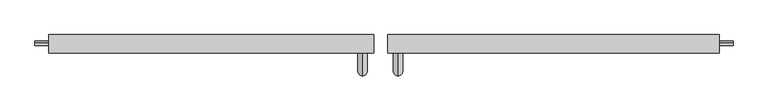
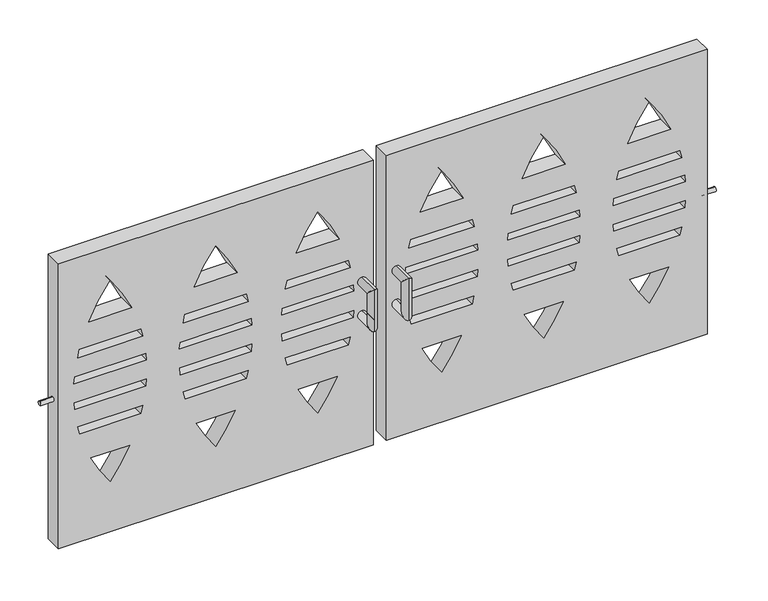
"""IFC4 building model written with IfcOpenShell, lengths in millimetres: proxy geometry."""

from ifc_helpers import new_model, si_unit, point, frame, frame_2d, origin, place, context, project, spatial, polyline, circle_curve, ellipse_curve, trimmed, segment, composite_curve, outline, extrude, source, transform, mapped, element, save
from ifc_brep_helpers import plane_surface, cylinder_surface, advanced_brep


def generic_models_477b0933(model_context):
    return source(origin(), model_context, "Body", "SolidModel", [
        extrude(outline(polyline([(0.0, 268.7654616), (1727.2, 268.7654616), (1727.2, -1534.6345384), (0.0, -1534.6345384), (0.0, 268.7654616)]), holes=[composite_curve([segment(trimmed(circle_curve(frame_2d((913.3858921, 735.2120442)), 991.7835907), [point((1315.7032602, -171.3062546))], [point((1522.0610264, -47.8264425))], True, "CARTESIAN"), True, "CONTINUOUS"), segment(trimmed(circle_curve(frame_2d((913.3858921, -830.8649293)), 991.7835907), [point((1522.0610264, -47.8264425))], [point((1315.7032602, 75.6533695))], True, "CARTESIAN"), True, "CONTINUOUS"), segment(polyline([(1315.7032602, 75.6533695), (1315.7032602, -171.3062546)]), True, "CONTINUOUS")], self_intersect=False), composite_curve([segment(trimmed(circle_curve(frame_2d((913.3858921, -830.8649293)), 991.7835907), [point((1167.7706197, 127.7398387))], [point((1120.5108318, 139.0494742))], True, "CARTESIAN"), True, "CONTINUOUS"), segment(polyline([(1120.5108318, 139.0494742), (1120.5108318, -234.7023593)]), True, "CONTINUOUS"), segment(trimmed(circle_curve(frame_2d((913.3858921, 735.2120442)), 991.7835907), [point((1120.5108318, -234.7023593))], [point((1167.7706197, -223.3927238))], True, "CARTESIAN"), True, "CONTINUOUS"), segment(polyline([(1167.7706197, -223.3927238), (1167.7706197, 127.7398387)]), True, "CONTINUOUS")], self_intersect=False), composite_curve([segment(trimmed(circle_curve(frame_2d((913.3858921, -830.8649293)), 991.7835907), [point((1008.9376367, 156.3050434))], [point((969.7809206, 159.3139897))], True, "CARTESIAN"), True, "CONTINUOUS"), segment(polyline([(969.7809206, 159.3139897), (969.7809206, -254.9668748)]), True, "CONTINUOUS"), segment(trimmed(circle_curve(frame_2d((913.3858921, 735.2120442)), 991.7835907), [point((969.7809206, -254.9668748))], [point((1008.9376367, -251.9579284))], True, "CARTESIAN"), True, "CONTINUOUS"), segment(polyline([(1008.9376367, -251.9579284), (1008.9376367, 156.3050434)]), True, "CONTINUOUS")], self_intersect=False), composite_curve([segment(trimmed(circle_curve(frame_2d((913.3858921, -830.8649293)), 991.7835907), [point((853.4628105, 159.1067446))], [point((811.4921317, 155.6706009))], True, "CARTESIAN"), True, "CONTINUOUS"), segment(polyline([(811.4921317, 155.6706009), (811.4921317, -251.323486)]), True, "CONTINUOUS"), segment(trimmed(circle_curve(frame_2d((913.3858921, 735.2120442)), 991.7835907), [point((811.4921317, -251.323486))], [point((853.4628105, -254.7596297))], True, "CARTESIAN"), True, "CONTINUOUS"), segment(polyline([(853.4628105, -254.7596297), (853.4628105, 159.1067446)]), True, "CONTINUOUS")], self_intersect=False), composite_curve([segment(trimmed(circle_curve(frame_2d((913.3858921, -830.8649293)), 991.7835907), [point((700.6764218, 137.8400681))], [point((655.683383, 126.8532483))], True, "CARTESIAN"), True, "CONTINUOUS"), segment(polyline([(655.683383, 126.8532483), (655.683383, -222.5061333)]), True, "CONTINUOUS"), segment(trimmed(circle_curve(frame_2d((913.3858921, 735.2120442)), 991.7835907), [point((655.683383, -222.5061333))], [point((700.6764218, -233.4929532))], True, "CARTESIAN"), True, "CONTINUOUS"), segment(polyline([(700.6764218, -233.4929532), (700.6764218, 137.8400681)]), True, "CONTINUOUS")], self_intersect=False), composite_curve([segment(trimmed(circle_curve(frame_2d((913.3858921, -830.8649293)), 991.7835907), [point((485.5755246, 63.9048625))], [point((304.7107578, -47.8264425))], True, "CARTESIAN"), True, "CONTINUOUS"), segment(trimmed(circle_curve(frame_2d((913.3858921, 735.2120442)), 991.7835907), [point((304.7107578, -47.8264425))], [point((485.5755246, -159.5577476))], True, "CARTESIAN"), True, "CONTINUOUS"), segment(polyline([(485.5755246, -159.5577476), (485.5755246, 63.9048625)]), True, "CONTINUOUS")], self_intersect=False), composite_curve([segment(polyline([(1315.7032602, -510.0774949), (1315.7032602, -757.0371191)]), True, "CONTINUOUS"), segment(trimmed(circle_curve(frame_2d((913.3858921, 149.4811798)), 991.7835907), [point((1315.7032602, -757.0371191))], [point((1522.0610264, -633.557307))], True, "CARTESIAN"), True, "CONTINUOUS"), segment(trimmed(circle_curve(frame_2d((913.3858921, -1416.5957937)), 991.7835907), [point((1522.0610264, -633.557307))], [point((1315.7032602, -510.0774949))], True, "CARTESIAN"), True, "CONTINUOUS")], self_intersect=False), composite_curve([segment(polyline([(1167.7706197, -809.1235882), (1167.7706197, -457.9910257)]), True, "CONTINUOUS"), segment(trimmed(circle_curve(frame_2d((913.3858921, -1416.5957937)), 991.7835907), [point((1167.7706197, -457.9910257))], [point((1120.5108318, -446.6813902))], True, "CARTESIAN"), True, "CONTINUOUS"), segment(polyline([(1120.5108318, -446.6813902), (1120.5108318, -820.4332237)]), True, "CONTINUOUS"), segment(trimmed(circle_curve(frame_2d((913.3858921, 149.4811798)), 991.7835907), [point((1120.5108318, -820.4332237))], [point((1167.7706197, -809.1235882))], True, "CARTESIAN"), True, "CONTINUOUS")], self_intersect=False), composite_curve([segment(polyline([(1008.9376367, -837.6887929), (1008.9376367, -429.4258211)]), True, "CONTINUOUS"), segment(trimmed(circle_curve(frame_2d((913.3858921, -1416.5957937)), 991.7835907), [point((1008.9376367, -429.4258211))], [point((969.7809206, -426.4168748))], True, "CARTESIAN"), True, "CONTINUOUS"), segment(polyline([(969.7809206, -426.4168748), (969.7809206, -840.6977392)]), True, "CONTINUOUS"), segment(trimmed(circle_curve(frame_2d((913.3858921, 149.4811798)), 991.7835907), [point((969.7809206, -840.6977392))], [point((1008.9376367, -837.6887929))], True, "CARTESIAN"), True, "CONTINUOUS")], self_intersect=False), composite_curve([segment(polyline([(853.4628105, -840.4904941), (853.4628105, -426.6241198)]), True, "CONTINUOUS"), segment(trimmed(circle_curve(frame_2d((913.3858921, -1416.5957937)), 991.7835907), [point((853.4628105, -426.6241198))], [point((811.4921317, -430.0602635))], True, "CARTESIAN"), True, "CONTINUOUS"), segment(polyline([(811.4921317, -430.0602635), (811.4921317, -837.0543504)]), True, "CONTINUOUS"), segment(trimmed(circle_curve(frame_2d((913.3858921, 149.4811798)), 991.7835907), [point((811.4921317, -837.0543504))], [point((853.4628105, -840.4904941))], True, "CARTESIAN"), True, "CONTINUOUS")], self_intersect=False), composite_curve([segment(polyline([(700.6764218, -819.2238176), (700.6764218, -447.8907963)]), True, "CONTINUOUS"), segment(trimmed(circle_curve(frame_2d((913.3858921, -1416.5957937)), 991.7835907), [point((700.6764218, -447.8907963))], [point((655.683383, -458.8776162))], True, "CARTESIAN"), True, "CONTINUOUS"), segment(polyline([(655.683383, -458.8776162), (655.683383, -808.2369978)]), True, "CONTINUOUS"), segment(trimmed(circle_curve(frame_2d((913.3858921, 149.4811798)), 991.7835907), [point((655.683383, -808.2369978))], [point((700.6764218, -819.2238176))], True, "CARTESIAN"), True, "CONTINUOUS")], self_intersect=False), composite_curve([segment(polyline([(485.5755246, -745.288612), (485.5755246, -521.8260019)]), True, "CONTINUOUS"), segment(trimmed(circle_curve(frame_2d((913.3858921, -1416.5957937)), 991.7835907), [point((485.5755246, -521.8260019))], [point((304.7107578, -633.557307))], True, "CARTESIAN"), True, "CONTINUOUS"), segment(trimmed(circle_curve(frame_2d((913.3858921, 149.4811798)), 991.7835907), [point((304.7107578, -633.557307))], [point((485.5755246, -745.288612))], True, "CARTESIAN"), True, "CONTINUOUS")], self_intersect=False), composite_curve([segment(trimmed(circle_curve(frame_2d((913.3858921, -455.2996847)), 991.7835907), [point((1315.7032602, -1361.8179835))], [point((1522.0610264, -1238.3381714))], True, "CARTESIAN"), True, "CONTINUOUS"), segment(trimmed(circle_curve(frame_2d((913.3858921, -2021.3766581)), 991.7835907), [point((1522.0610264, -1238.3381714))], [point((1315.7032602, -1114.8583593))], True, "CARTESIAN"), True, "CONTINUOUS"), segment(polyline([(1315.7032602, -1114.8583593), (1315.7032602, -1361.8179835)]), True, "CONTINUOUS")], self_intersect=False), composite_curve([segment(trimmed(circle_curve(frame_2d((913.3858921, -2021.3766581)), 991.7835907), [point((1167.7706197, -1062.7718902))], [point((1120.5108318, -1051.4622546))], True, "CARTESIAN"), True, "CONTINUOUS"), segment(polyline([(1120.5108318, -1051.4622546), (1120.5108318, -1425.2140882)]), True, "CONTINUOUS"), segment(trimmed(circle_curve(frame_2d((913.3858921, -455.2996847)), 991.7835907), [point((1120.5108318, -1425.2140882))], [point((1167.7706197, -1413.9044526))], True, "CARTESIAN"), True, "CONTINUOUS"), segment(polyline([(1167.7706197, -1413.9044526), (1167.7706197, -1062.7718902)]), True, "CONTINUOUS")], self_intersect=False), composite_curve([segment(trimmed(circle_curve(frame_2d((913.3858921, -2021.3766581)), 991.7835907), [point((1008.9376367, -1034.2066855))], [point((969.7809206, -1031.1977392))], True, "CARTESIAN"), True, "CONTINUOUS"), segment(polyline([(969.7809206, -1031.1977392), (969.7809206, -1445.4786036)]), True, "CONTINUOUS"), segment(trimmed(circle_curve(frame_2d((913.3858921, -455.2996847)), 991.7835907), [point((969.7809206, -1445.4786036))], [point((1008.9376367, -1442.4696573))], True, "CARTESIAN"), True, "CONTINUOUS"), segment(polyline([(1008.9376367, -1442.4696573), (1008.9376367, -1034.2066855)]), True, "CONTINUOUS")], self_intersect=False), composite_curve([segment(trimmed(circle_curve(frame_2d((913.3858921, -2021.3766581)), 991.7835907), [point((853.4628105, -1031.4049843))], [point((811.4921317, -1034.8411279))], True, "CARTESIAN"), True, "CONTINUOUS"), segment(polyline([(811.4921317, -1034.8411279), (811.4921317, -1441.8352149)]), True, "CONTINUOUS"), segment(trimmed(circle_curve(frame_2d((913.3858921, -455.2996847)), 991.7835907), [point((811.4921317, -1441.8352149))], [point((853.4628105, -1445.2713585))], True, "CARTESIAN"), True, "CONTINUOUS"), segment(polyline([(853.4628105, -1445.2713585), (853.4628105, -1031.4049843)]), True, "CONTINUOUS")], self_intersect=False), composite_curve([segment(trimmed(circle_curve(frame_2d((913.3858921, -2021.3766581)), 991.7835907), [point((700.6764218, -1052.6716607))], [point((655.683383, -1063.6584806))], True, "CARTESIAN"), True, "CONTINUOUS"), segment(polyline([(655.683383, -1063.6584806), (655.683383, -1413.0178622)]), True, "CONTINUOUS"), segment(trimmed(circle_curve(frame_2d((913.3858921, -455.2996847)), 991.7835907), [point((655.683383, -1413.0178622))], [point((700.6764218, -1424.0046821))], True, "CARTESIAN"), True, "CONTINUOUS"), segment(polyline([(700.6764218, -1424.0046821), (700.6764218, -1052.6716607)]), True, "CONTINUOUS")], self_intersect=False), composite_curve([segment(trimmed(circle_curve(frame_2d((913.3858921, -2021.3766581)), 991.7835907), [point((485.5755246, -1126.6068664))], [point((304.7107578, -1238.3381714))], True, "CARTESIAN"), True, "CONTINUOUS"), segment(trimmed(circle_curve(frame_2d((913.3858921, -455.2996847)), 991.7835907), [point((304.7107578, -1238.3381714))], [point((485.5755246, -1350.0694764))], True, "CARTESIAN"), True, "CONTINUOUS"), segment(polyline([(485.5755246, -1350.0694764), (485.5755246, -1126.6068664)]), True, "CONTINUOUS")], self_intersect=False)]), frame((0.0, -101.6, 0.0), z_axis=(0.0, 1.0, 0.0), x_axis=(0.0, 0.0, 1.0)), (0.0, 0.0, 1.0), 101.6),
        extrude(outline(polyline([(1727.2, 2183.266195), (1727.2, 344.9654616), (0.0, 344.9654616), (0.0, 2183.266195), (1727.2, 2183.266195)]), holes=[composite_curve([segment(polyline([(1315.7032602, 785.0371778), (1315.7032602, 538.0775536)]), True, "CONTINUOUS"), segment(trimmed(circle_curve(frame_2d((913.3858921, 1444.5958525)), 991.7835907), [point((1315.7032602, 538.0775536))], [point((1522.0610264, 661.5573657))], True, "CARTESIAN"), True, "CONTINUOUS"), segment(trimmed(circle_curve(frame_2d((913.3858921, -121.481121)), 991.7835907), [point((1522.0610264, 661.5573657))], [point((1315.7032602, 785.0371778))], True, "CARTESIAN"), True, "CONTINUOUS")], self_intersect=False), composite_curve([segment(polyline([(1167.7706197, 485.9910845), (1167.7706197, 837.1236469)]), True, "CONTINUOUS"), segment(trimmed(circle_curve(frame_2d((913.3858921, -121.481121)), 991.7835907), [point((1167.7706197, 837.1236469))], [point((1120.5108318, 848.4332825))], True, "CARTESIAN"), True, "CONTINUOUS"), segment(polyline([(1120.5108318, 848.4332825), (1120.5108318, 474.681449)]), True, "CONTINUOUS"), segment(trimmed(circle_curve(frame_2d((913.3858921, 1444.5958525)), 991.7835907), [point((1120.5108318, 474.681449))], [point((1167.7706197, 485.9910845))], True, "CARTESIAN"), True, "CONTINUOUS")], self_intersect=False), composite_curve([segment(polyline([(1008.9376367, 457.4258798), (1008.9376367, 865.6888516)]), True, "CONTINUOUS"), segment(trimmed(circle_curve(frame_2d((913.3858921, -121.481121)), 991.7835907), [point((1008.9376367, 865.6888516))], [point((969.7809206, 868.6977979))], True, "CARTESIAN"), True, "CONTINUOUS"), segment(polyline([(969.7809206, 868.6977979), (969.7809206, 454.4169335)]), True, "CONTINUOUS"), segment(trimmed(circle_curve(frame_2d((913.3858921, 1444.5958525)), 991.7835907), [point((969.7809206, 454.4169335))], [point((1008.9376367, 457.4258798))], True, "CARTESIAN"), True, "CONTINUOUS")], self_intersect=False), composite_curve([segment(polyline([(853.4628105, 454.6241786), (853.4628105, 868.4905529)]), True, "CONTINUOUS"), segment(trimmed(circle_curve(frame_2d((913.3858921, -121.481121)), 991.7835907), [point((853.4628105, 868.4905529))], [point((811.4921317, 865.0544092))], True, "CARTESIAN"), True, "CONTINUOUS"), segment(polyline([(811.4921317, 865.0544092), (811.4921317, 458.0603222)]), True, "CONTINUOUS"), segment(trimmed(circle_curve(frame_2d((913.3858921, 1444.5958525)), 991.7835907), [point((811.4921317, 458.0603222))], [point((853.4628105, 454.6241786))], True, "CARTESIAN"), True, "CONTINUOUS")], self_intersect=False), composite_curve([segment(polyline([(700.6764218, 475.890855), (700.6764218, 847.2238764)]), True, "CONTINUOUS"), segment(trimmed(circle_curve(frame_2d((913.3858921, -121.481121)), 991.7835907), [point((700.6764218, 847.2238764))], [point((655.683383, 836.2370565))], True, "CARTESIAN"), True, "CONTINUOUS"), segment(polyline([(655.683383, 836.2370565), (655.683383, 486.8776749)]), True, "CONTINUOUS"), segment(trimmed(circle_curve(frame_2d((913.3858921, 1444.5958525)), 991.7835907), [point((655.683383, 486.8776749))], [point((700.6764218, 475.890855))], True, "CARTESIAN"), True, "CONTINUOUS")], self_intersect=False), composite_curve([segment(polyline([(485.5755246, 549.8260607), (485.5755246, 773.2886707)]), True, "CONTINUOUS"), segment(trimmed(circle_curve(frame_2d((913.3858921, -121.481121)), 991.7835907), [point((485.5755246, 773.2886707))], [point((304.7107578, 661.5573657))], True, "CARTESIAN"), True, "CONTINUOUS"), segment(trimmed(circle_curve(frame_2d((913.3858921, 1444.5958525)), 991.7835907), [point((304.7107578, 661.5573657))], [point((485.5755246, 549.8260607))], True, "CARTESIAN"), True, "CONTINUOUS")], self_intersect=False), composite_curve([segment(trimmed(circle_curve(frame_2d((913.3858921, 2030.3267169)), 991.7835907), [point((1315.7032602, 1123.8084181))], [point((1522.0610264, 1247.2882301))], True, "CARTESIAN"), True, "CONTINUOUS"), segment(trimmed(circle_curve(frame_2d((913.3858921, 464.2497434)), 991.7835907), [point((1522.0610264, 1247.2882301))], [point((1315.7032602, 1370.7680422))], True, "CARTESIAN"), True, "CONTINUOUS"), segment(polyline([(1315.7032602, 1370.7680422), (1315.7032602, 1123.8084181)]), True, "CONTINUOUS")], self_intersect=False), composite_curve([segment(trimmed(circle_curve(frame_2d((913.3858921, 464.2497434)), 991.7835907), [point((1167.7706197, 1422.8545114))], [point((1120.5108318, 1434.1641469))], True, "CARTESIAN"), True, "CONTINUOUS"), segment(polyline([(1120.5108318, 1434.1641469), (1120.5108318, 1060.4123134)]), True, "CONTINUOUS"), segment(trimmed(circle_curve(frame_2d((913.3858921, 2030.3267169)), 991.7835907), [point((1120.5108318, 1060.4123134))], [point((1167.7706197, 1071.7219489))], True, "CARTESIAN"), True, "CONTINUOUS"), segment(polyline([(1167.7706197, 1071.7219489), (1167.7706197, 1422.8545114)]), True, "CONTINUOUS")], self_intersect=False), composite_curve([segment(trimmed(circle_curve(frame_2d((913.3858921, 464.2497434)), 991.7835907), [point((1008.9376367, 1451.419716))], [point((969.7809206, 1454.4286624))], True, "CARTESIAN"), True, "CONTINUOUS"), segment(polyline([(969.7809206, 1454.4286624), (969.7809206, 1040.1477979)]), True, "CONTINUOUS"), segment(trimmed(circle_curve(frame_2d((913.3858921, 2030.3267169)), 991.7835907), [point((969.7809206, 1040.1477979))], [point((1008.9376367, 1043.1567442))], True, "CARTESIAN"), True, "CONTINUOUS"), segment(polyline([(1008.9376367, 1043.1567442), (1008.9376367, 1451.419716)]), True, "CONTINUOUS")], self_intersect=False), composite_curve([segment(trimmed(circle_curve(frame_2d((913.3858921, 464.2497434)), 991.7835907), [point((853.4628105, 1454.2214173))], [point((811.4921317, 1450.7852736))], True, "CARTESIAN"), True, "CONTINUOUS"), segment(polyline([(811.4921317, 1450.7852736), (811.4921317, 1043.7911867)]), True, "CONTINUOUS"), segment(trimmed(circle_curve(frame_2d((913.3858921, 2030.3267169)), 991.7835907), [point((811.4921317, 1043.7911867))], [point((853.4628105, 1040.355043))], True, "CARTESIAN"), True, "CONTINUOUS"), segment(polyline([(853.4628105, 1040.355043), (853.4628105, 1454.2214173)]), True, "CONTINUOUS")], self_intersect=False), composite_curve([segment(trimmed(circle_curve(frame_2d((913.3858921, 464.2497434)), 991.7835907), [point((700.6764218, 1432.9547408))], [point((655.683383, 1421.9679209))], True, "CARTESIAN"), True, "CONTINUOUS"), segment(polyline([(655.683383, 1421.9679209), (655.683383, 1072.6085394)]), True, "CONTINUOUS"), segment(trimmed(circle_curve(frame_2d((913.3858921, 2030.3267169)), 991.7835907), [point((655.683383, 1072.6085394))], [point((700.6764218, 1061.6217195))], True, "CARTESIAN"), True, "CONTINUOUS"), segment(polyline([(700.6764218, 1061.6217195), (700.6764218, 1432.9547408)]), True, "CONTINUOUS")], self_intersect=False), composite_curve([segment(trimmed(circle_curve(frame_2d((913.3858921, 464.2497434)), 991.7835907), [point((485.5755246, 1359.0195352))], [point((304.7107578, 1247.2882301))], True, "CARTESIAN"), True, "CONTINUOUS"), segment(trimmed(circle_curve(frame_2d((913.3858921, 2030.3267169)), 991.7835907), [point((304.7107578, 1247.2882301))], [point((485.5755246, 1135.5569251))], True, "CARTESIAN"), True, "CONTINUOUS"), segment(polyline([(485.5755246, 1135.5569251), (485.5755246, 1359.0195352)]), True, "CONTINUOUS")], self_intersect=False), composite_curve([segment(polyline([(1315.7032602, 1975.5489067), (1315.7032602, 1728.5892825)]), True, "CONTINUOUS"), segment(trimmed(circle_curve(frame_2d((913.3858921, 2635.1075813)), 991.7835907), [point((1315.7032602, 1728.5892825))], [point((1522.0610264, 1852.0690946))], True, "CARTESIAN"), True, "CONTINUOUS"), segment(trimmed(circle_curve(frame_2d((913.3858921, 1069.0306078)), 991.7835907), [point((1522.0610264, 1852.0690946))], [point((1315.7032602, 1975.5489067))], True, "CARTESIAN"), True, "CONTINUOUS")], self_intersect=False), composite_curve([segment(polyline([(1167.7706197, 1676.5028134), (1167.7706197, 2027.6353758)]), True, "CONTINUOUS"), segment(trimmed(circle_curve(frame_2d((913.3858921, 1069.0306078)), 991.7835907), [point((1167.7706197, 2027.6353758))], [point((1120.5108318, 2038.9450113))], True, "CARTESIAN"), True, "CONTINUOUS"), segment(polyline([(1120.5108318, 2038.9450113), (1120.5108318, 1665.1931778)]), True, "CONTINUOUS"), segment(trimmed(circle_curve(frame_2d((913.3858921, 2635.1075813)), 991.7835907), [point((1120.5108318, 1665.1931778))], [point((1167.7706197, 1676.5028134))], True, "CARTESIAN"), True, "CONTINUOUS")], self_intersect=False), composite_curve([segment(polyline([(1008.9376367, 1647.9376087), (1008.9376367, 2056.2005805)]), True, "CONTINUOUS"), segment(trimmed(circle_curve(frame_2d((913.3858921, 1069.0306078)), 991.7835907), [point((1008.9376367, 2056.2005805))], [point((969.7809206, 2059.2095268))], True, "CARTESIAN"), True, "CONTINUOUS"), segment(polyline([(969.7809206, 2059.2095268), (969.7809206, 1644.9286624)]), True, "CONTINUOUS"), segment(trimmed(circle_curve(frame_2d((913.3858921, 2635.1075813)), 991.7835907), [point((969.7809206, 1644.9286624))], [point((1008.9376367, 1647.9376087))], True, "CARTESIAN"), True, "CONTINUOUS")], self_intersect=False), composite_curve([segment(polyline([(853.4628105, 1645.1359074), (853.4628105, 2059.0022817)]), True, "CONTINUOUS"), segment(trimmed(circle_curve(frame_2d((913.3858921, 1069.0306078)), 991.7835907), [point((853.4628105, 2059.0022817))], [point((811.4921317, 2055.566138))], True, "CARTESIAN"), True, "CONTINUOUS"), segment(polyline([(811.4921317, 2055.566138), (811.4921317, 1648.5720511)]), True, "CONTINUOUS"), segment(trimmed(circle_curve(frame_2d((913.3858921, 2635.1075813)), 991.7835907), [point((811.4921317, 1648.5720511))], [point((853.4628105, 1645.1359074))], True, "CARTESIAN"), True, "CONTINUOUS")], self_intersect=False), composite_curve([segment(polyline([(700.6764218, 1666.4025839), (700.6764218, 2037.7356052)]), True, "CONTINUOUS"), segment(trimmed(circle_curve(frame_2d((913.3858921, 1069.0306078)), 991.7835907), [point((700.6764218, 2037.7356052))], [point((655.683383, 2026.7487854))], True, "CARTESIAN"), True, "CONTINUOUS"), segment(polyline([(655.683383, 2026.7487854), (655.683383, 1677.3894038)]), True, "CONTINUOUS"), segment(trimmed(circle_curve(frame_2d((913.3858921, 2635.1075813)), 991.7835907), [point((655.683383, 1677.3894038))], [point((700.6764218, 1666.4025839))], True, "CARTESIAN"), True, "CONTINUOUS")], self_intersect=False), composite_curve([segment(polyline([(485.5755246, 1740.3377895), (485.5755246, 1963.8003996)]), True, "CONTINUOUS"), segment(trimmed(circle_curve(frame_2d((913.3858921, 1069.0306078)), 991.7835907), [point((485.5755246, 1963.8003996))], [point((304.7107578, 1852.0690946))], True, "CARTESIAN"), True, "CONTINUOUS"), segment(trimmed(circle_curve(frame_2d((913.3858921, 2635.1075813)), 991.7835907), [point((304.7107578, 1852.0690946))], [point((485.5755246, 1740.3377895))], True, "CARTESIAN"), True, "CONTINUOUS")], self_intersect=False)]), frame((0.0, -101.6, 0.0), z_axis=(0.0, 1.0, 0.0), x_axis=(0.0, 0.0, 1.0)), (0.0, 0.0, 1.0), 101.6),
        advanced_brep(
        [(205.2654616, -101.6, 1039.4610264), (205.2654616, -101.6, 988.6610264), (205.2654616, -101.6, 785.4610264), (205.2654616, -101.6, 836.2610264), (205.2654616, -228.6, 1039.4610264), (205.2654616, -177.8, 988.6610264), (205.2654616, -228.6, 785.4610264), (205.2654616, -177.8, 836.2610264)],
        [
            (0, 1, circle_curve(frame((205.2654616, -101.6, 1014.0610264), z_axis=(0.0, 1.0, 0.0), x_axis=(0.0, 0.0, -1.0)), 25.4)),
            (1, 0, circle_curve(frame((205.2654616, -101.6, 1014.0610264), z_axis=(0.0, 1.0, 0.0), x_axis=(0.0, 0.0, -1.0)), 25.4)),
            (2, 3, circle_curve(frame((205.2654616, -101.6, 810.8610264), z_axis=(0.0, 1.0, 0.0), x_axis=(0.0, 0.0, 1.0)), 25.4)),
            (3, 2, circle_curve(frame((205.2654616, -101.6, 810.8610264), z_axis=(0.0, 1.0, 0.0), x_axis=(0.0, 0.0, 1.0)), 25.4)),
            (0, 4),
            (4, 5, ellipse_curve(frame((205.2654616, -203.2, 1014.0610264), z_axis=(0.0, 0.7071067811865495, 0.7071067811865455), x_axis=(0.0, 0.7071067811865457, -0.7071067811865493)), 35.9210245, 25.4)),
            (5, 1),
            (5, 4, ellipse_curve(frame((205.2654616, -203.2, 1014.0610264), z_axis=(0.0, 0.7071067811865495, 0.7071067811865455), x_axis=(0.0, 0.7071067811865457, -0.7071067811865493)), 35.9210245, 25.4)),
            (4, 6),
            (6, 7, ellipse_curve(frame((205.2654616, -203.2, 810.8610264), z_axis=(0.0, -0.7071067811865457, 0.7071067811865495), x_axis=(0.0, 0.7071067811865496, 0.7071067811865455)), 35.9210245, 25.4)),
            (7, 5),
            (7, 6, ellipse_curve(frame((205.2654616, -203.2, 810.8610264), z_axis=(0.0, -0.7071067811865457, 0.7071067811865495), x_axis=(0.0, 0.7071067811865496, 0.7071067811865455)), 35.9210245, 25.4)),
            (6, 2),
            (3, 7),
        ],
        [
            plane_surface(frame((205.2654616, -101.6, 1014.0610264), z_axis=(0.0, 1.0, 0.0), x_axis=(1.0, 0.0, 0.0))),
            plane_surface(frame((205.2654616, -101.6, 810.8610264), z_axis=(0.0, 1.0, 0.0), x_axis=(1.0, 0.0, 0.0))),
            cylinder_surface(frame((205.2654616, -101.6, 1014.0610264), z_axis=(0.0, 1.0, 0.0), x_axis=(0.0, 0.0, -1.0)), 25.4),
            cylinder_surface(frame((205.2654616, -203.2, 1014.0610264), z_axis=(0.0, 0.0, 1.0), x_axis=(0.0, 1.0, 0.0)), 25.4),
            cylinder_surface(frame((205.2654616, -203.2, 810.8610264), z_axis=(0.0, -1.0, 0.0), x_axis=(0.0, 0.0, 1.0)), 25.4),
        ],
        [
            (0, [[1, 2]]),
            (1, [[3, 4]]),
            (2, [[-1, 5, 6, 7]]),
            (2, [[-2, -7, 8, -5]]),
            (3, [[-6, 9, 10, 11]]),
            (3, [[-8, -11, 12, -9]]),
            (4, [[-10, 13, -4, 14]]),
            (4, [[-12, -14, -3, -13]]),
        ],
    ),
        advanced_brep(
        [(402.1154616, -101.6, 1039.4610264), (402.1154616, -101.6, 988.6610264), (402.1154616, -101.6, 785.4610264), (402.1154616, -101.6, 836.2610264), (402.1154616, -228.6, 1039.4610264), (402.1154616, -177.8, 988.6610264), (402.1154616, -228.6, 785.4610264), (402.1154616, -177.8, 836.2610264)],
        [
            (0, 1, circle_curve(frame((402.1154616, -101.6, 1014.0610264), z_axis=(0.0, 1.0, 0.0), x_axis=(0.0, 0.0, -1.0)), 25.4)),
            (1, 0, circle_curve(frame((402.1154616, -101.6, 1014.0610264), z_axis=(0.0, 1.0, 0.0), x_axis=(0.0, 0.0, -1.0)), 25.4)),
            (2, 3, circle_curve(frame((402.1154616, -101.6, 810.8610264), z_axis=(0.0, 1.0, 0.0), x_axis=(0.0, 0.0, 1.0)), 25.4)),
            (3, 2, circle_curve(frame((402.1154616, -101.6, 810.8610264), z_axis=(0.0, 1.0, 0.0), x_axis=(0.0, 0.0, 1.0)), 25.4)),
            (0, 4),
            (4, 5, ellipse_curve(frame((402.1154616, -203.2, 1014.0610264), z_axis=(0.0, 0.7071067811865495, 0.7071067811865455), x_axis=(0.0, 0.7071067811865457, -0.7071067811865493)), 35.9210245, 25.4)),
            (5, 1),
            (5, 4, ellipse_curve(frame((402.1154616, -203.2, 1014.0610264), z_axis=(0.0, 0.7071067811865495, 0.7071067811865455), x_axis=(0.0, 0.7071067811865457, -0.7071067811865493)), 35.9210245, 25.4)),
            (4, 6),
            (6, 7, ellipse_curve(frame((402.1154616, -203.2, 810.8610264), z_axis=(0.0, -0.7071067811865457, 0.7071067811865495), x_axis=(0.0, 0.7071067811865496, 0.7071067811865455)), 35.9210245, 25.4)),
            (7, 5),
            (7, 6, ellipse_curve(frame((402.1154616, -203.2, 810.8610264), z_axis=(0.0, -0.7071067811865457, 0.7071067811865495), x_axis=(0.0, 0.7071067811865496, 0.7071067811865455)), 35.9210245, 25.4)),
            (6, 2),
            (3, 7),
        ],
        [
            plane_surface(frame((402.1154616, -101.6, 1014.0610264), z_axis=(0.0, 1.0, 0.0), x_axis=(1.0, 0.0, 0.0))),
            plane_surface(frame((402.1154616, -101.6, 810.8610264), z_axis=(0.0, 1.0, 0.0), x_axis=(1.0, 0.0, 0.0))),
            cylinder_surface(frame((402.1154616, -101.6, 1014.0610264), z_axis=(0.0, 1.0, 0.0), x_axis=(0.0, 0.0, -1.0)), 25.4),
            cylinder_surface(frame((402.1154616, -203.2, 1014.0610264), z_axis=(0.0, 0.0, 1.0), x_axis=(0.0, 1.0, 0.0)), 25.4),
            cylinder_surface(frame((402.1154616, -203.2, 810.8610264), z_axis=(0.0, -1.0, 0.0), x_axis=(0.0, 0.0, 1.0)), 25.4),
        ],
        [
            (0, [[1, 2]]),
            (1, [[3, 4]]),
            (2, [[-1, 5, 6, 7]]),
            (2, [[-2, -7, 8, -5]]),
            (3, [[-6, 9, 10, 11]]),
            (3, [[-8, -11, 12, -9]]),
            (4, [[-10, 13, -4, 14]]),
            (4, [[-12, -14, -3, -13]]),
        ],
    ),
        extrude(outline(composite_curve([segment(trimmed(circle_curve(frame_2d((-47.1865605, 821.1501685)), 12.7), [point((-47.1865605, 833.8501685))], [point((-47.1865605, 808.4501685))], False, "CARTESIAN"), True, "CONTINUOUS"), segment(trimmed(circle_curve(frame_2d((-47.1865605, 821.1501685)), 12.7), [point((-47.1865605, 808.4501685))], [point((-47.1865605, 833.8501685))], False, "CARTESIAN"), True, "CONTINUOUS")], self_intersect=False)), frame((2183.266195, 0.0, 0.0), z_axis=(1.0, 0.0, 0.0), x_axis=(0.0, 1.0, 0.0)), (0.0, 0.0, 1.0), 76.2),
        extrude(outline(composite_curve([segment(trimmed(circle_curve(frame_2d((-47.1865605, 876.3)), 12.7), [point((-47.1865605, 889.0))], [point((-47.1865605, 863.6))], False, "CARTESIAN"), True, "CONTINUOUS"), segment(trimmed(circle_curve(frame_2d((-47.1865605, 876.3)), 12.7), [point((-47.1865605, 863.6))], [point((-47.1865605, 889.0))], False, "CARTESIAN"), True, "CONTINUOUS")], self_intersect=False)), frame((-1610.8345384, 0.0, 0.0), z_axis=(1.0, 0.0, 0.0), x_axis=(0.0, 1.0, 0.0)), (0.0, 0.0, 1.0), 76.2),
    ])


if __name__ == "__main__":
    model = new_model("IFC4")
    model_context = context("Model", 3, world=origin())
    ifc_project = project(units=[si_unit("LENGTHUNIT", "METRE", prefix="MILLI")], contexts=[model_context])
    site = spatial("IfcSite", under=ifc_project)
    building = spatial("IfcBuilding", under=site)
    placement = place(None, origin())
    generic_models_shape = generic_models_477b0933(model_context)
    element("IfcBuildingElementProxy", 1, Name="Generic Models", at=placement, inside=building, context=model_context, shape_type="MappedRepresentation", body=[
        mapped(generic_models_shape, transform((0.0, 0.0, 0.0), x_axis=(1.0, 0.0, 0.0), y_axis=(0.0, 1.0, 0.0), z_axis=(0.0, 0.0, 1.0))),
    ])
    save(model, "model.ifc")

# Revit data of these elements
# Type
#   Default Elevation = 0
